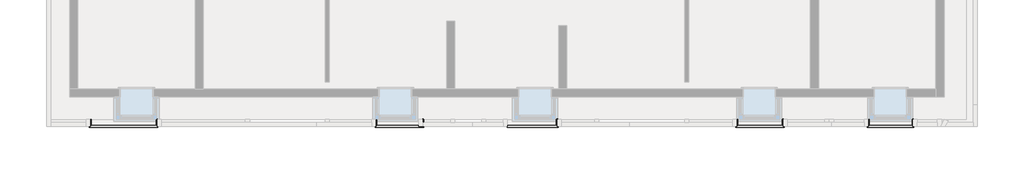
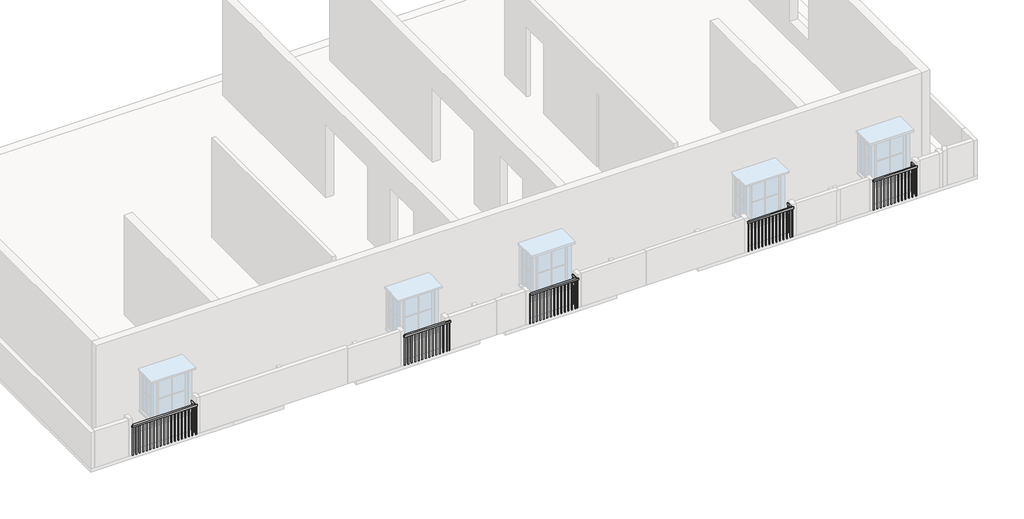
# One storey, part 3 of 7: 5 railings.
"""IFC4 building model written with IfcOpenShell, lengths in millimetres."""

from ifc_helpers import new_model, si_unit, frame, origin, place, context, project, spatial, polyline, outline, extrude, faceted_brep, element, save

model = new_model("IFC4")

# Units and contexts
model_context = context("Model", 3, world=origin())
ifc_project = project(units=[si_unit("LENGTHUNIT", "METRE", prefix="MILLI")], contexts=[model_context])

# Site, building, storey
site = spatial("IfcSite", under=ifc_project)
building = spatial("IfcBuilding", under=site)
storey = spatial("IfcBuildingStorey", under=building, Elevation=3200.4)

# Railings
placement = place(None, origin())
element("IfcRailing", 1, ObjectType="Handrail - Rectangular", at=placement, inside=storey, context=model_context, shape_type="SolidModel", body=[
    faceted_brep([(-11856.9067989, -4623.6932193, 4114.8), (-11856.9067989, -4623.6932193, 4064.0), (-11907.7067989, -4623.6932193, 4064.0), (-11907.7067989, -4623.6932193, 4114.8), (-11856.9067989, -4801.4932661, 4114.8), (-11856.9067989, -4801.4932661, 4064.0), (-11907.7067989, -4852.2932661, 4064.0), (-11907.7067989, -4852.2932661, 4114.8), (-10071.3470335, -4801.4932661, 4114.8), (-10071.3470335, -4801.4932661, 4064.0), (-10020.5470335, -4852.2932661, 4064.0), (-10020.5470335, -4852.2932661, 4114.8), (-10071.3470335, -4623.6932193, 4114.8), (-10020.5470335, -4623.6932193, 4114.8), (-10020.5470335, -4623.6932193, 4064.0), (-10071.3470335, -4623.6932193, 4064.0)], [[[0, 1, 2, 3]], [[1, 0, 4, 5]], [[2, 1, 5, 6]], [[3, 2, 6, 7]], [[0, 3, 7, 4]], [[5, 4, 8, 9]], [[6, 5, 9, 10]], [[7, 6, 10, 11]], [[4, 7, 11, 8]], [[12, 13, 14, 15]], [[9, 8, 12, 15]], [[10, 9, 15, 14]], [[11, 10, 14, 13]], [[8, 11, 13, 12]]]),
    extrude(outline(polyline([(-10036.4220335, -4633.2182661), (-10055.4720335, -4633.2182661), (-10055.4720335, -4614.1682661), (-10036.4220335, -4614.1682661), (-10036.4220335, -4633.2182661)])), frame((0.0, 0.0, 3200.4), z_axis=(0.0, 0.0, 1.0), x_axis=(1.0, 0.0, 0.0)), (0.0, 0.0, 1.0), 863.6),
    extrude(outline(polyline([(-10036.4220335, -4734.8182661), (-10055.4720335, -4734.8182661), (-10055.4720335, -4715.7682661), (-10036.4220335, -4715.7682661), (-10036.4220335, -4734.8182661)])), frame((0.0, 0.0, 3200.4), z_axis=(0.0, 0.0, 1.0), x_axis=(1.0, 0.0, 0.0)), (0.0, 0.0, 1.0), 863.6),
    extrude(outline(polyline([(-10063.0317989, -4836.4182661), (-10063.0317989, -4817.3682661), (-10043.9817989, -4817.3682661), (-10043.9817989, -4836.4182661), (-10063.0317989, -4836.4182661)])), frame((0.0, 0.0, 3200.4), z_axis=(0.0, 0.0, 1.0), x_axis=(1.0, 0.0, 0.0)), (0.0, 0.0, 1.0), 863.6),
    extrude(outline(polyline([(-10164.6317989, -4836.4182661), (-10164.6317989, -4817.3682661), (-10145.5817989, -4817.3682661), (-10145.5817989, -4836.4182661), (-10164.6317989, -4836.4182661)])), frame((0.0, 0.0, 3200.4), z_axis=(0.0, 0.0, 1.0), x_axis=(1.0, 0.0, 0.0)), (0.0, 0.0, 1.0), 863.6),
    extrude(outline(polyline([(-10266.2317989, -4836.4182661), (-10266.2317989, -4817.3682661), (-10247.1817989, -4817.3682661), (-10247.1817989, -4836.4182661), (-10266.2317989, -4836.4182661)])), frame((0.0, 0.0, 3200.4), z_axis=(0.0, 0.0, 1.0), x_axis=(1.0, 0.0, 0.0)), (0.0, 0.0, 1.0), 863.6),
    extrude(outline(polyline([(-10367.8317989, -4836.4182661), (-10367.8317989, -4817.3682661), (-10348.7817989, -4817.3682661), (-10348.7817989, -4836.4182661), (-10367.8317989, -4836.4182661)])), frame((0.0, 0.0, 3200.4), z_axis=(0.0, 0.0, 1.0), x_axis=(1.0, 0.0, 0.0)), (0.0, 0.0, 1.0), 863.6),
    extrude(outline(polyline([(-10469.4317989, -4836.4182661), (-10469.4317989, -4817.3682661), (-10450.3817989, -4817.3682661), (-10450.3817989, -4836.4182661), (-10469.4317989, -4836.4182661)])), frame((0.0, 0.0, 3200.4), z_axis=(0.0, 0.0, 1.0), x_axis=(1.0, 0.0, 0.0)), (0.0, 0.0, 1.0), 863.6),
    extrude(outline(polyline([(-10571.0317989, -4836.4182661), (-10571.0317989, -4817.3682661), (-10551.9817989, -4817.3682661), (-10551.9817989, -4836.4182661), (-10571.0317989, -4836.4182661)])), frame((0.0, 0.0, 3200.4), z_axis=(0.0, 0.0, 1.0), x_axis=(1.0, 0.0, 0.0)), (0.0, 0.0, 1.0), 863.6),
    extrude(outline(polyline([(-10672.6317989, -4836.4182661), (-10672.6317989, -4817.3682661), (-10653.5817989, -4817.3682661), (-10653.5817989, -4836.4182661), (-10672.6317989, -4836.4182661)])), frame((0.0, 0.0, 3200.4), z_axis=(0.0, 0.0, 1.0), x_axis=(1.0, 0.0, 0.0)), (0.0, 0.0, 1.0), 863.6),
    extrude(outline(polyline([(-10774.2317989, -4836.4182661), (-10774.2317989, -4817.3682661), (-10755.1817989, -4817.3682661), (-10755.1817989, -4836.4182661), (-10774.2317989, -4836.4182661)])), frame((0.0, 0.0, 3200.4), z_axis=(0.0, 0.0, 1.0), x_axis=(1.0, 0.0, 0.0)), (0.0, 0.0, 1.0), 863.6),
    extrude(outline(polyline([(-10875.8317989, -4836.4182661), (-10875.8317989, -4817.3682661), (-10856.7817989, -4817.3682661), (-10856.7817989, -4836.4182661), (-10875.8317989, -4836.4182661)])), frame((0.0, 0.0, 3200.4), z_axis=(0.0, 0.0, 1.0), x_axis=(1.0, 0.0, 0.0)), (0.0, 0.0, 1.0), 863.6),
    extrude(outline(polyline([(-10977.4317989, -4836.4182661), (-10977.4317989, -4817.3682661), (-10958.3817989, -4817.3682661), (-10958.3817989, -4836.4182661), (-10977.4317989, -4836.4182661)])), frame((0.0, 0.0, 3200.4), z_axis=(0.0, 0.0, 1.0), x_axis=(1.0, 0.0, 0.0)), (0.0, 0.0, 1.0), 863.6),
    extrude(outline(polyline([(-11079.0317989, -4836.4182661), (-11079.0317989, -4817.3682661), (-11059.9817989, -4817.3682661), (-11059.9817989, -4836.4182661), (-11079.0317989, -4836.4182661)])), frame((0.0, 0.0, 3200.4), z_axis=(0.0, 0.0, 1.0), x_axis=(1.0, 0.0, 0.0)), (0.0, 0.0, 1.0), 863.6),
    extrude(outline(polyline([(-11180.6317989, -4836.4182661), (-11180.6317989, -4817.3682661), (-11161.5817989, -4817.3682661), (-11161.5817989, -4836.4182661), (-11180.6317989, -4836.4182661)])), frame((0.0, 0.0, 3200.4), z_axis=(0.0, 0.0, 1.0), x_axis=(1.0, 0.0, 0.0)), (0.0, 0.0, 1.0), 863.6),
    extrude(outline(polyline([(-11282.2317989, -4836.4182661), (-11282.2317989, -4817.3682661), (-11263.1817989, -4817.3682661), (-11263.1817989, -4836.4182661), (-11282.2317989, -4836.4182661)])), frame((0.0, 0.0, 3200.4), z_axis=(0.0, 0.0, 1.0), x_axis=(1.0, 0.0, 0.0)), (0.0, 0.0, 1.0), 863.6),
    extrude(outline(polyline([(-11383.8317989, -4836.4182661), (-11383.8317989, -4817.3682661), (-11364.7817989, -4817.3682661), (-11364.7817989, -4836.4182661), (-11383.8317989, -4836.4182661)])), frame((0.0, 0.0, 3200.4), z_axis=(0.0, 0.0, 1.0), x_axis=(1.0, 0.0, 0.0)), (0.0, 0.0, 1.0), 863.6),
    extrude(outline(polyline([(-11485.4317989, -4836.4182661), (-11485.4317989, -4817.3682661), (-11466.3817989, -4817.3682661), (-11466.3817989, -4836.4182661), (-11485.4317989, -4836.4182661)])), frame((0.0, 0.0, 3200.4), z_axis=(0.0, 0.0, 1.0), x_axis=(1.0, 0.0, 0.0)), (0.0, 0.0, 1.0), 863.6),
    extrude(outline(polyline([(-11587.0317989, -4836.4182661), (-11587.0317989, -4817.3682661), (-11567.9817989, -4817.3682661), (-11567.9817989, -4836.4182661), (-11587.0317989, -4836.4182661)])), frame((0.0, 0.0, 3200.4), z_axis=(0.0, 0.0, 1.0), x_axis=(1.0, 0.0, 0.0)), (0.0, 0.0, 1.0), 863.6),
    extrude(outline(polyline([(-11688.6317989, -4836.4182661), (-11688.6317989, -4817.3682661), (-11669.5817989, -4817.3682661), (-11669.5817989, -4836.4182661), (-11688.6317989, -4836.4182661)])), frame((0.0, 0.0, 3200.4), z_axis=(0.0, 0.0, 1.0), x_axis=(1.0, 0.0, 0.0)), (0.0, 0.0, 1.0), 863.6),
    extrude(outline(polyline([(-11790.2317989, -4836.4182661), (-11790.2317989, -4817.3682661), (-11771.1817989, -4817.3682661), (-11771.1817989, -4836.4182661), (-11790.2317989, -4836.4182661)])), frame((0.0, 0.0, 3200.4), z_axis=(0.0, 0.0, 1.0), x_axis=(1.0, 0.0, 0.0)), (0.0, 0.0, 1.0), 863.6),
    extrude(outline(polyline([(-11891.8317989, -4817.3682193), (-11872.7817989, -4817.3682193), (-11872.7817989, -4836.4182193), (-11891.8317989, -4836.4182193), (-11891.8317989, -4817.3682193)])), frame((0.0, 0.0, 3200.4), z_axis=(0.0, 0.0, 1.0), x_axis=(1.0, 0.0, 0.0)), (0.0, 0.0, 1.0), 863.6),
    extrude(outline(polyline([(-11891.8317989, -4715.7682193), (-11872.7817989, -4715.7682193), (-11872.7817989, -4734.8182193), (-11891.8317989, -4734.8182193), (-11891.8317989, -4715.7682193)])), frame((0.0, 0.0, 3200.4), z_axis=(0.0, 0.0, 1.0), x_axis=(1.0, 0.0, 0.0)), (0.0, 0.0, 1.0), 863.6),
    extrude(outline(polyline([(-10055.4720335, -4836.4182661), (-10055.4720335, -4817.3682661), (-10036.4220335, -4817.3682661), (-10036.4220335, -4836.4182661), (-10055.4720335, -4836.4182661)])), frame((0.0, 0.0, 3200.4), z_axis=(0.0, 0.0, 1.0), x_axis=(1.0, 0.0, 0.0)), (0.0, 0.0, 1.0), 863.6),
    extrude(outline(polyline([(-11891.8317989, -4817.3682661), (-11872.7817989, -4817.3682661), (-11872.7817989, -4836.4182661), (-11891.8317989, -4836.4182661), (-11891.8317989, -4817.3682661)])), frame((0.0, 0.0, 3200.4), z_axis=(0.0, 0.0, 1.0), x_axis=(1.0, 0.0, 0.0)), (0.0, 0.0, 1.0), 863.6),
    extrude(outline(polyline([(-10036.4220335, -4642.7432193), (-10055.4720335, -4642.7432193), (-10055.4720335, -4623.6932193), (-10036.4220335, -4623.6932193), (-10036.4220335, -4642.7432193)])), frame((0.0, 0.0, 3200.4), z_axis=(0.0, 0.0, 1.0), x_axis=(1.0, 0.0, 0.0)), (0.0, 0.0, 1.0), 863.6),
    extrude(outline(polyline([(-11891.8317989, -4623.6932193), (-11872.7817989, -4623.6932193), (-11872.7817989, -4642.7432193), (-11891.8317989, -4642.7432193), (-11891.8317989, -4623.6932193)])), frame((0.0, 0.0, 3200.4), z_axis=(0.0, 0.0, 1.0), x_axis=(1.0, 0.0, 0.0)), (0.0, 0.0, 1.0), 863.6),
])
element("IfcRailing", 2, ObjectType="Handrail - Rectangular", at=placement, inside=storey, context=model_context, shape_type="SolidModel", body=[
    faceted_brep([(-3995.0987995, -4623.6932193, 4114.8), (-3995.0987995, -4623.6932193, 4064.0), (-4045.8987995, -4623.6932193, 4064.0), (-4045.8987995, -4623.6932193, 4114.8), (-3995.0987995, -4801.4932661, 4114.8), (-3995.0987995, -4801.4932661, 4064.0), (-4045.8987995, -4852.2932661, 4064.0), (-4045.8987995, -4852.2932661, 4114.8), (-2750.4987995, -4801.4932661, 4114.8), (-2750.4987995, -4801.4932661, 4064.0), (-2699.6987995, -4852.2932661, 4064.0), (-2699.6987995, -4852.2932661, 4114.8), (-2750.4987995, -4623.6932193, 4114.8), (-2699.6987995, -4623.6932193, 4114.8), (-2699.6987995, -4623.6932193, 4064.0), (-2750.4987995, -4623.6932193, 4064.0)], [[[0, 1, 2, 3]], [[1, 0, 4, 5]], [[2, 1, 5, 6]], [[3, 2, 6, 7]], [[0, 3, 7, 4]], [[5, 4, 8, 9]], [[6, 5, 9, 10]], [[7, 6, 10, 11]], [[4, 7, 11, 8]], [[12, 13, 14, 15]], [[9, 8, 12, 15]], [[10, 9, 15, 14]], [[11, 10, 14, 13]], [[8, 11, 13, 12]]]),
    extrude(outline(polyline([(-2715.5737995, -4633.2182661), (-2734.6237995, -4633.2182661), (-2734.6237995, -4614.1682661), (-2715.5737995, -4614.1682661), (-2715.5737995, -4633.2182661)])), frame((0.0, 0.0, 3200.4), z_axis=(0.0, 0.0, 1.0), x_axis=(1.0, 0.0, 0.0)), (0.0, 0.0, 1.0), 863.6),
    extrude(outline(polyline([(-2715.5737995, -4734.8182661), (-2734.6237995, -4734.8182661), (-2734.6237995, -4715.7682661), (-2715.5737995, -4715.7682661), (-2715.5737995, -4734.8182661)])), frame((0.0, 0.0, 3200.4), z_axis=(0.0, 0.0, 1.0), x_axis=(1.0, 0.0, 0.0)), (0.0, 0.0, 1.0), 863.6),
    extrude(outline(polyline([(-2810.8237995, -4836.4182661), (-2810.8237995, -4817.3682661), (-2791.7737995, -4817.3682661), (-2791.7737995, -4836.4182661), (-2810.8237995, -4836.4182661)])), frame((0.0, 0.0, 3200.4), z_axis=(0.0, 0.0, 1.0), x_axis=(1.0, 0.0, 0.0)), (0.0, 0.0, 1.0), 863.6),
    extrude(outline(polyline([(-2912.4237995, -4836.4182661), (-2912.4237995, -4817.3682661), (-2893.3737995, -4817.3682661), (-2893.3737995, -4836.4182661), (-2912.4237995, -4836.4182661)])), frame((0.0, 0.0, 3200.4), z_axis=(0.0, 0.0, 1.0), x_axis=(1.0, 0.0, 0.0)), (0.0, 0.0, 1.0), 863.6),
    extrude(outline(polyline([(-3014.0237995, -4836.4182661), (-3014.0237995, -4817.3682661), (-2994.9737995, -4817.3682661), (-2994.9737995, -4836.4182661), (-3014.0237995, -4836.4182661)])), frame((0.0, 0.0, 3200.4), z_axis=(0.0, 0.0, 1.0), x_axis=(1.0, 0.0, 0.0)), (0.0, 0.0, 1.0), 863.6),
    extrude(outline(polyline([(-3115.6237995, -4836.4182661), (-3115.6237995, -4817.3682661), (-3096.5737995, -4817.3682661), (-3096.5737995, -4836.4182661), (-3115.6237995, -4836.4182661)])), frame((0.0, 0.0, 3200.4), z_axis=(0.0, 0.0, 1.0), x_axis=(1.0, 0.0, 0.0)), (0.0, 0.0, 1.0), 863.6),
    extrude(outline(polyline([(-3217.2237995, -4836.4182661), (-3217.2237995, -4817.3682661), (-3198.1737995, -4817.3682661), (-3198.1737995, -4836.4182661), (-3217.2237995, -4836.4182661)])), frame((0.0, 0.0, 3200.4), z_axis=(0.0, 0.0, 1.0), x_axis=(1.0, 0.0, 0.0)), (0.0, 0.0, 1.0), 863.6),
    extrude(outline(polyline([(-3318.8237995, -4836.4182661), (-3318.8237995, -4817.3682661), (-3299.7737995, -4817.3682661), (-3299.7737995, -4836.4182661), (-3318.8237995, -4836.4182661)])), frame((0.0, 0.0, 3200.4), z_axis=(0.0, 0.0, 1.0), x_axis=(1.0, 0.0, 0.0)), (0.0, 0.0, 1.0), 863.6),
    extrude(outline(polyline([(-3420.4237995, -4836.4182661), (-3420.4237995, -4817.3682661), (-3401.3737995, -4817.3682661), (-3401.3737995, -4836.4182661), (-3420.4237995, -4836.4182661)])), frame((0.0, 0.0, 3200.4), z_axis=(0.0, 0.0, 1.0), x_axis=(1.0, 0.0, 0.0)), (0.0, 0.0, 1.0), 863.6),
    extrude(outline(polyline([(-3522.0237995, -4836.4182661), (-3522.0237995, -4817.3682661), (-3502.9737995, -4817.3682661), (-3502.9737995, -4836.4182661), (-3522.0237995, -4836.4182661)])), frame((0.0, 0.0, 3200.4), z_axis=(0.0, 0.0, 1.0), x_axis=(1.0, 0.0, 0.0)), (0.0, 0.0, 1.0), 863.6),
    extrude(outline(polyline([(-3623.6237995, -4836.4182661), (-3623.6237995, -4817.3682661), (-3604.5737995, -4817.3682661), (-3604.5737995, -4836.4182661), (-3623.6237995, -4836.4182661)])), frame((0.0, 0.0, 3200.4), z_axis=(0.0, 0.0, 1.0), x_axis=(1.0, 0.0, 0.0)), (0.0, 0.0, 1.0), 863.6),
    extrude(outline(polyline([(-3725.2237995, -4836.4182661), (-3725.2237995, -4817.3682661), (-3706.1737995, -4817.3682661), (-3706.1737995, -4836.4182661), (-3725.2237995, -4836.4182661)])), frame((0.0, 0.0, 3200.4), z_axis=(0.0, 0.0, 1.0), x_axis=(1.0, 0.0, 0.0)), (0.0, 0.0, 1.0), 863.6),
    extrude(outline(polyline([(-3826.8237995, -4836.4182661), (-3826.8237995, -4817.3682661), (-3807.7737995, -4817.3682661), (-3807.7737995, -4836.4182661), (-3826.8237995, -4836.4182661)])), frame((0.0, 0.0, 3200.4), z_axis=(0.0, 0.0, 1.0), x_axis=(1.0, 0.0, 0.0)), (0.0, 0.0, 1.0), 863.6),
    extrude(outline(polyline([(-3928.4237995, -4836.4182661), (-3928.4237995, -4817.3682661), (-3909.3737995, -4817.3682661), (-3909.3737995, -4836.4182661), (-3928.4237995, -4836.4182661)])), frame((0.0, 0.0, 3200.4), z_axis=(0.0, 0.0, 1.0), x_axis=(1.0, 0.0, 0.0)), (0.0, 0.0, 1.0), 863.6),
    extrude(outline(polyline([(-4030.0237995, -4817.3682193), (-4010.9737995, -4817.3682193), (-4010.9737995, -4836.4182193), (-4030.0237995, -4836.4182193), (-4030.0237995, -4817.3682193)])), frame((0.0, 0.0, 3200.4), z_axis=(0.0, 0.0, 1.0), x_axis=(1.0, 0.0, 0.0)), (0.0, 0.0, 1.0), 863.6),
    extrude(outline(polyline([(-4030.0237995, -4715.7682193), (-4010.9737995, -4715.7682193), (-4010.9737995, -4734.8182193), (-4030.0237995, -4734.8182193), (-4030.0237995, -4715.7682193)])), frame((0.0, 0.0, 3200.4), z_axis=(0.0, 0.0, 1.0), x_axis=(1.0, 0.0, 0.0)), (0.0, 0.0, 1.0), 863.6),
    extrude(outline(polyline([(-2734.6237995, -4836.4182661), (-2734.6237995, -4817.3682661), (-2715.5737995, -4817.3682661), (-2715.5737995, -4836.4182661), (-2734.6237995, -4836.4182661)])), frame((0.0, 0.0, 3200.4), z_axis=(0.0, 0.0, 1.0), x_axis=(1.0, 0.0, 0.0)), (0.0, 0.0, 1.0), 863.6),
    extrude(outline(polyline([(-4030.0237995, -4817.3682661), (-4010.9737995, -4817.3682661), (-4010.9737995, -4836.4182661), (-4030.0237995, -4836.4182661), (-4030.0237995, -4817.3682661)])), frame((0.0, 0.0, 3200.4), z_axis=(0.0, 0.0, 1.0), x_axis=(1.0, 0.0, 0.0)), (0.0, 0.0, 1.0), 863.6),
    extrude(outline(polyline([(-2715.5737995, -4642.7432193), (-2734.6237995, -4642.7432193), (-2734.6237995, -4623.6932193), (-2715.5737995, -4623.6932193), (-2715.5737995, -4642.7432193)])), frame((0.0, 0.0, 3200.4), z_axis=(0.0, 0.0, 1.0), x_axis=(1.0, 0.0, 0.0)), (0.0, 0.0, 1.0), 863.6),
    extrude(outline(polyline([(-4030.0237995, -4623.6932193), (-4010.9737995, -4623.6932193), (-4010.9737995, -4642.7432193), (-4030.0237995, -4642.7432193), (-4030.0237995, -4623.6932193)])), frame((0.0, 0.0, 3200.4), z_axis=(0.0, 0.0, 1.0), x_axis=(1.0, 0.0, 0.0)), (0.0, 0.0, 1.0), 863.6),
])
element("IfcRailing", 3, ObjectType="Handrail - Rectangular", at=placement, inside=storey, context=model_context, shape_type="SolidModel", body=[
    faceted_brep([(-406.2065315, -4801.4932661, 4114.8), (-406.2065315, -4801.4932661, 4064.0), (-406.2065315, -4852.2932661, 4064.0), (-406.2065315, -4852.2932661, 4114.8), (944.6932011, -4801.4932661, 4114.8), (944.6932011, -4801.4932661, 4064.0), (995.4932011, -4852.2932661, 4064.0), (995.4932011, -4852.2932661, 4114.8), (944.6932011, -4623.6932193, 4114.8), (995.4932011, -4623.6932193, 4114.8), (995.4932011, -4623.6932193, 4064.0), (944.6932011, -4623.6932193, 4064.0)], [[[0, 1, 2, 3]], [[1, 0, 4, 5]], [[2, 1, 5, 6]], [[3, 2, 6, 7]], [[0, 3, 7, 4]], [[8, 9, 10, 11]], [[5, 4, 8, 11]], [[6, 5, 11, 10]], [[7, 6, 10, 9]], [[4, 7, 9, 8]]]),
    extrude(outline(polyline([(979.6182011, -4633.2182661), (960.5682011, -4633.2182661), (960.5682011, -4614.1682661), (979.6182011, -4614.1682661), (979.6182011, -4633.2182661)])), frame((0.0, 0.0, 3200.4), z_axis=(0.0, 0.0, 1.0), x_axis=(1.0, 0.0, 0.0)), (0.0, 0.0, 1.0), 863.6),
    extrude(outline(polyline([(979.6182011, -4734.8182661), (960.5682011, -4734.8182661), (960.5682011, -4715.7682661), (979.6182011, -4715.7682661), (979.6182011, -4734.8182661)])), frame((0.0, 0.0, 3200.4), z_axis=(0.0, 0.0, 1.0), x_axis=(1.0, 0.0, 0.0)), (0.0, 0.0, 1.0), 863.6),
    extrude(outline(polyline([(905.0684685, -4836.4182661), (905.0684685, -4817.3682661), (924.1184685, -4817.3682661), (924.1184685, -4836.4182661), (905.0684685, -4836.4182661)])), frame((0.0, 0.0, 3200.4), z_axis=(0.0, 0.0, 1.0), x_axis=(1.0, 0.0, 0.0)), (0.0, 0.0, 1.0), 863.6),
    extrude(outline(polyline([(803.4684685, -4836.4182661), (803.4684685, -4817.3682661), (822.5184685, -4817.3682661), (822.5184685, -4836.4182661), (803.4684685, -4836.4182661)])), frame((0.0, 0.0, 3200.4), z_axis=(0.0, 0.0, 1.0), x_axis=(1.0, 0.0, 0.0)), (0.0, 0.0, 1.0), 863.6),
    extrude(outline(polyline([(701.8684685, -4836.4182661), (701.8684685, -4817.3682661), (720.9184685, -4817.3682661), (720.9184685, -4836.4182661), (701.8684685, -4836.4182661)])), frame((0.0, 0.0, 3200.4), z_axis=(0.0, 0.0, 1.0), x_axis=(1.0, 0.0, 0.0)), (0.0, 0.0, 1.0), 863.6),
    extrude(outline(polyline([(600.2684685, -4836.4182661), (600.2684685, -4817.3682661), (619.3184685, -4817.3682661), (619.3184685, -4836.4182661), (600.2684685, -4836.4182661)])), frame((0.0, 0.0, 3200.4), z_axis=(0.0, 0.0, 1.0), x_axis=(1.0, 0.0, 0.0)), (0.0, 0.0, 1.0), 863.6),
    extrude(outline(polyline([(498.6684685, -4836.4182661), (498.6684685, -4817.3682661), (517.7184685, -4817.3682661), (517.7184685, -4836.4182661), (498.6684685, -4836.4182661)])), frame((0.0, 0.0, 3200.4), z_axis=(0.0, 0.0, 1.0), x_axis=(1.0, 0.0, 0.0)), (0.0, 0.0, 1.0), 863.6),
    extrude(outline(polyline([(397.0684685, -4836.4182661), (397.0684685, -4817.3682661), (416.1184685, -4817.3682661), (416.1184685, -4836.4182661), (397.0684685, -4836.4182661)])), frame((0.0, 0.0, 3200.4), z_axis=(0.0, 0.0, 1.0), x_axis=(1.0, 0.0, 0.0)), (0.0, 0.0, 1.0), 863.6),
    extrude(outline(polyline([(295.4684685, -4836.4182661), (295.4684685, -4817.3682661), (314.5184685, -4817.3682661), (314.5184685, -4836.4182661), (295.4684685, -4836.4182661)])), frame((0.0, 0.0, 3200.4), z_axis=(0.0, 0.0, 1.0), x_axis=(1.0, 0.0, 0.0)), (0.0, 0.0, 1.0), 863.6),
    extrude(outline(polyline([(193.8684685, -4836.4182661), (193.8684685, -4817.3682661), (212.9184685, -4817.3682661), (212.9184685, -4836.4182661), (193.8684685, -4836.4182661)])), frame((0.0, 0.0, 3200.4), z_axis=(0.0, 0.0, 1.0), x_axis=(1.0, 0.0, 0.0)), (0.0, 0.0, 1.0), 863.6),
    extrude(outline(polyline([(92.2684685, -4836.4182661), (92.2684685, -4817.3682661), (111.3184685, -4817.3682661), (111.3184685, -4836.4182661), (92.2684685, -4836.4182661)])), frame((0.0, 0.0, 3200.4), z_axis=(0.0, 0.0, 1.0), x_axis=(1.0, 0.0, 0.0)), (0.0, 0.0, 1.0), 863.6),
    extrude(outline(polyline([(-9.3315315, -4836.4182661), (-9.3315315, -4817.3682661), (9.7184685, -4817.3682661), (9.7184685, -4836.4182661), (-9.3315315, -4836.4182661)])), frame((0.0, 0.0, 3200.4), z_axis=(0.0, 0.0, 1.0), x_axis=(1.0, 0.0, 0.0)), (0.0, 0.0, 1.0), 863.6),
    extrude(outline(polyline([(-110.9315315, -4836.4182661), (-110.9315315, -4817.3682661), (-91.8815315, -4817.3682661), (-91.8815315, -4836.4182661), (-110.9315315, -4836.4182661)])), frame((0.0, 0.0, 3200.4), z_axis=(0.0, 0.0, 1.0), x_axis=(1.0, 0.0, 0.0)), (0.0, 0.0, 1.0), 863.6),
    extrude(outline(polyline([(-212.5315315, -4836.4182661), (-212.5315315, -4817.3682661), (-193.4815315, -4817.3682661), (-193.4815315, -4836.4182661), (-212.5315315, -4836.4182661)])), frame((0.0, 0.0, 3200.4), z_axis=(0.0, 0.0, 1.0), x_axis=(1.0, 0.0, 0.0)), (0.0, 0.0, 1.0), 863.6),
    extrude(outline(polyline([(-314.1315315, -4836.4182661), (-314.1315315, -4817.3682661), (-295.0815315, -4817.3682661), (-295.0815315, -4836.4182661), (-314.1315315, -4836.4182661)])), frame((0.0, 0.0, 3200.4), z_axis=(0.0, 0.0, 1.0), x_axis=(1.0, 0.0, 0.0)), (0.0, 0.0, 1.0), 863.6),
    extrude(outline(polyline([(960.5682011, -4836.4182661), (960.5682011, -4817.3682661), (979.6182011, -4817.3682661), (979.6182011, -4836.4182661), (960.5682011, -4836.4182661)])), frame((0.0, 0.0, 3200.4), z_axis=(0.0, 0.0, 1.0), x_axis=(1.0, 0.0, 0.0)), (0.0, 0.0, 1.0), 863.6),
    extrude(outline(polyline([(979.6182011, -4642.7432193), (960.5682011, -4642.7432193), (960.5682011, -4623.6932193), (979.6182011, -4623.6932193), (979.6182011, -4642.7432193)])), frame((0.0, 0.0, 3200.4), z_axis=(0.0, 0.0, 1.0), x_axis=(1.0, 0.0, 0.0)), (0.0, 0.0, 1.0), 863.6),
    extrude(outline(polyline([(-406.2065315, -4836.4182661), (-406.2065315, -4817.3682661), (-387.1565315, -4817.3682661), (-387.1565315, -4836.4182661), (-406.2065315, -4836.4182661)])), frame((0.0, 0.0, 3200.4), z_axis=(0.0, 0.0, 1.0), x_axis=(1.0, 0.0, 0.0)), (0.0, 0.0, 1.0), 863.6),
])
element("IfcRailing", 4, ObjectType="Handrail - Rectangular", at=placement, inside=storey, context=model_context, shape_type="SolidModel", body=[
    faceted_brep([(5942.6512082, -4623.6932193, 4114.8), (5942.6512082, -4623.6932193, 4064.0), (5891.8512082, -4623.6932193, 4064.0), (5891.8512082, -4623.6932193, 4114.8), (5942.6512082, -4801.4932661, 4114.8), (5942.6512082, -4801.4932661, 4064.0), (5891.8512082, -4852.2932661, 4064.0), (5891.8512082, -4852.2932661, 4114.8), (7164.9011643, -4801.4932661, 4114.8), (7164.9011643, -4801.4932661, 4064.0), (7215.7011643, -4852.2932661, 4064.0), (7215.7011643, -4852.2932661, 4114.8), (7164.9011643, -4623.6932193, 4114.8), (7215.7011643, -4623.6932193, 4114.8), (7215.7011643, -4623.6932193, 4064.0), (7164.9011643, -4623.6932193, 4064.0)], [[[0, 1, 2, 3]], [[1, 0, 4, 5]], [[2, 1, 5, 6]], [[3, 2, 6, 7]], [[0, 3, 7, 4]], [[5, 4, 8, 9]], [[6, 5, 9, 10]], [[7, 6, 10, 11]], [[4, 7, 11, 8]], [[12, 13, 14, 15]], [[9, 8, 12, 15]], [[10, 9, 15, 14]], [[11, 10, 14, 13]], [[8, 11, 13, 12]]]),
    extrude(outline(polyline([(7199.8261643, -4633.2182661), (7180.7761643, -4633.2182661), (7180.7761643, -4614.1682661), (7199.8261643, -4614.1682661), (7199.8261643, -4633.2182661)])), frame((0.0, 0.0, 3200.4), z_axis=(0.0, 0.0, 1.0), x_axis=(1.0, 0.0, 0.0)), (0.0, 0.0, 1.0), 863.6),
    extrude(outline(polyline([(7199.8261643, -4734.8182661), (7180.7761643, -4734.8182661), (7180.7761643, -4715.7682661), (7199.8261643, -4715.7682661), (7199.8261643, -4734.8182661)])), frame((0.0, 0.0, 3200.4), z_axis=(0.0, 0.0, 1.0), x_axis=(1.0, 0.0, 0.0)), (0.0, 0.0, 1.0), 863.6),
    extrude(outline(polyline([(7126.9262082, -4836.4182661), (7126.9262082, -4817.3682661), (7145.9762082, -4817.3682661), (7145.9762082, -4836.4182661), (7126.9262082, -4836.4182661)])), frame((0.0, 0.0, 3200.4), z_axis=(0.0, 0.0, 1.0), x_axis=(1.0, 0.0, 0.0)), (0.0, 0.0, 1.0), 863.6),
    extrude(outline(polyline([(7025.3262082, -4836.4182661), (7025.3262082, -4817.3682661), (7044.3762082, -4817.3682661), (7044.3762082, -4836.4182661), (7025.3262082, -4836.4182661)])), frame((0.0, 0.0, 3200.4), z_axis=(0.0, 0.0, 1.0), x_axis=(1.0, 0.0, 0.0)), (0.0, 0.0, 1.0), 863.6),
    extrude(outline(polyline([(6923.7262082, -4836.4182661), (6923.7262082, -4817.3682661), (6942.7762082, -4817.3682661), (6942.7762082, -4836.4182661), (6923.7262082, -4836.4182661)])), frame((0.0, 0.0, 3200.4), z_axis=(0.0, 0.0, 1.0), x_axis=(1.0, 0.0, 0.0)), (0.0, 0.0, 1.0), 863.6),
    extrude(outline(polyline([(6822.1262082, -4836.4182661), (6822.1262082, -4817.3682661), (6841.1762082, -4817.3682661), (6841.1762082, -4836.4182661), (6822.1262082, -4836.4182661)])), frame((0.0, 0.0, 3200.4), z_axis=(0.0, 0.0, 1.0), x_axis=(1.0, 0.0, 0.0)), (0.0, 0.0, 1.0), 863.6),
    extrude(outline(polyline([(6720.5262082, -4836.4182661), (6720.5262082, -4817.3682661), (6739.5762082, -4817.3682661), (6739.5762082, -4836.4182661), (6720.5262082, -4836.4182661)])), frame((0.0, 0.0, 3200.4), z_axis=(0.0, 0.0, 1.0), x_axis=(1.0, 0.0, 0.0)), (0.0, 0.0, 1.0), 863.6),
    extrude(outline(polyline([(6618.9262082, -4836.4182661), (6618.9262082, -4817.3682661), (6637.9762082, -4817.3682661), (6637.9762082, -4836.4182661), (6618.9262082, -4836.4182661)])), frame((0.0, 0.0, 3200.4), z_axis=(0.0, 0.0, 1.0), x_axis=(1.0, 0.0, 0.0)), (0.0, 0.0, 1.0), 863.6),
    extrude(outline(polyline([(6517.3262082, -4836.4182661), (6517.3262082, -4817.3682661), (6536.3762082, -4817.3682661), (6536.3762082, -4836.4182661), (6517.3262082, -4836.4182661)])), frame((0.0, 0.0, 3200.4), z_axis=(0.0, 0.0, 1.0), x_axis=(1.0, 0.0, 0.0)), (0.0, 0.0, 1.0), 863.6),
    extrude(outline(polyline([(6415.7262082, -4836.4182661), (6415.7262082, -4817.3682661), (6434.7762082, -4817.3682661), (6434.7762082, -4836.4182661), (6415.7262082, -4836.4182661)])), frame((0.0, 0.0, 3200.4), z_axis=(0.0, 0.0, 1.0), x_axis=(1.0, 0.0, 0.0)), (0.0, 0.0, 1.0), 863.6),
    extrude(outline(polyline([(6314.1262082, -4836.4182661), (6314.1262082, -4817.3682661), (6333.1762082, -4817.3682661), (6333.1762082, -4836.4182661), (6314.1262082, -4836.4182661)])), frame((0.0, 0.0, 3200.4), z_axis=(0.0, 0.0, 1.0), x_axis=(1.0, 0.0, 0.0)), (0.0, 0.0, 1.0), 863.6),
    extrude(outline(polyline([(6212.5262082, -4836.4182661), (6212.5262082, -4817.3682661), (6231.5762082, -4817.3682661), (6231.5762082, -4836.4182661), (6212.5262082, -4836.4182661)])), frame((0.0, 0.0, 3200.4), z_axis=(0.0, 0.0, 1.0), x_axis=(1.0, 0.0, 0.0)), (0.0, 0.0, 1.0), 863.6),
    extrude(outline(polyline([(6110.9262082, -4836.4182661), (6110.9262082, -4817.3682661), (6129.9762082, -4817.3682661), (6129.9762082, -4836.4182661), (6110.9262082, -4836.4182661)])), frame((0.0, 0.0, 3200.4), z_axis=(0.0, 0.0, 1.0), x_axis=(1.0, 0.0, 0.0)), (0.0, 0.0, 1.0), 863.6),
    extrude(outline(polyline([(6009.3262082, -4836.4182661), (6009.3262082, -4817.3682661), (6028.3762082, -4817.3682661), (6028.3762082, -4836.4182661), (6009.3262082, -4836.4182661)])), frame((0.0, 0.0, 3200.4), z_axis=(0.0, 0.0, 1.0), x_axis=(1.0, 0.0, 0.0)), (0.0, 0.0, 1.0), 863.6),
    extrude(outline(polyline([(5907.7262082, -4817.3682193), (5926.7762082, -4817.3682193), (5926.7762082, -4836.4182193), (5907.7262082, -4836.4182193), (5907.7262082, -4817.3682193)])), frame((0.0, 0.0, 3200.4), z_axis=(0.0, 0.0, 1.0), x_axis=(1.0, 0.0, 0.0)), (0.0, 0.0, 1.0), 863.6),
    extrude(outline(polyline([(5907.7262082, -4715.7682193), (5926.7762082, -4715.7682193), (5926.7762082, -4734.8182193), (5907.7262082, -4734.8182193), (5907.7262082, -4715.7682193)])), frame((0.0, 0.0, 3200.4), z_axis=(0.0, 0.0, 1.0), x_axis=(1.0, 0.0, 0.0)), (0.0, 0.0, 1.0), 863.6),
    extrude(outline(polyline([(7180.7761643, -4836.4182661), (7180.7761643, -4817.3682661), (7199.8261643, -4817.3682661), (7199.8261643, -4836.4182661), (7180.7761643, -4836.4182661)])), frame((0.0, 0.0, 3200.4), z_axis=(0.0, 0.0, 1.0), x_axis=(1.0, 0.0, 0.0)), (0.0, 0.0, 1.0), 863.6),
    extrude(outline(polyline([(5907.7262082, -4817.3682661), (5926.7762082, -4817.3682661), (5926.7762082, -4836.4182661), (5907.7262082, -4836.4182661), (5907.7262082, -4817.3682661)])), frame((0.0, 0.0, 3200.4), z_axis=(0.0, 0.0, 1.0), x_axis=(1.0, 0.0, 0.0)), (0.0, 0.0, 1.0), 863.6),
    extrude(outline(polyline([(7199.8261643, -4642.7432193), (7180.7761643, -4642.7432193), (7180.7761643, -4623.6932193), (7199.8261643, -4623.6932193), (7199.8261643, -4642.7432193)])), frame((0.0, 0.0, 3200.4), z_axis=(0.0, 0.0, 1.0), x_axis=(1.0, 0.0, 0.0)), (0.0, 0.0, 1.0), 863.6),
    extrude(outline(polyline([(5907.7262082, -4623.6932193), (5926.7762082, -4623.6932193), (5926.7762082, -4642.7432193), (5907.7262082, -4642.7432193), (5907.7262082, -4623.6932193)])), frame((0.0, 0.0, 3200.4), z_axis=(0.0, 0.0, 1.0), x_axis=(1.0, 0.0, 0.0)), (0.0, 0.0, 1.0), 863.6),
])
element("IfcRailing", 5, ObjectType="Handrail - Rectangular", at=placement, inside=storey, context=model_context, shape_type="SolidModel", body=[
    faceted_brep([(9562.1512082, -4623.6932193, 4114.8), (9562.1512082, -4623.6932193, 4064.0), (9511.3512082, -4623.6932193, 4064.0), (9511.3512082, -4623.6932193, 4114.8), (9562.1512082, -4801.4932661, 4114.8), (9562.1512082, -4801.4932661, 4064.0), (9511.3512082, -4852.2932661, 4064.0), (9511.3512082, -4852.2932661, 4114.8), (10738.7617205, -4801.4932661, 4114.8), (10738.7617205, -4801.4932661, 4064.0), (10789.5617205, -4852.2932661, 4064.0), (10789.5617205, -4852.2932661, 4114.8), (10738.7617205, -4623.6932193, 4114.8), (10789.5617205, -4623.6932193, 4114.8), (10789.5617205, -4623.6932193, 4064.0), (10738.7617205, -4623.6932193, 4064.0)], [[[0, 1, 2, 3]], [[1, 0, 4, 5]], [[2, 1, 5, 6]], [[3, 2, 6, 7]], [[0, 3, 7, 4]], [[5, 4, 8, 9]], [[6, 5, 9, 10]], [[7, 6, 10, 11]], [[4, 7, 11, 8]], [[12, 13, 14, 15]], [[9, 8, 12, 15]], [[10, 9, 15, 14]], [[11, 10, 14, 13]], [[8, 11, 13, 12]]]),
    extrude(outline(polyline([(10754.6367205, -4633.2182661), (10754.6367205, -4614.1682661), (10773.6867205, -4614.1682661), (10773.6867205, -4633.2182661), (10754.6367205, -4633.2182661)])), frame((0.0, 0.0, 3200.4), z_axis=(0.0, 0.0, 1.0), x_axis=(1.0, 0.0, 0.0)), (0.0, 0.0, 1.0), 863.6),
    extrude(outline(polyline([(10754.6367205, -4734.8182661), (10754.6367205, -4715.7682661), (10773.6867205, -4715.7682661), (10773.6867205, -4734.8182661), (10754.6367205, -4734.8182661)])), frame((0.0, 0.0, 3200.4), z_axis=(0.0, 0.0, 1.0), x_axis=(1.0, 0.0, 0.0)), (0.0, 0.0, 1.0), 863.6),
    extrude(outline(polyline([(10746.4262082, -4817.3682661), (10765.4762082, -4817.3682661), (10765.4762082, -4836.4182661), (10746.4262082, -4836.4182661), (10746.4262082, -4817.3682661)])), frame((0.0, 0.0, 3200.4), z_axis=(0.0, 0.0, 1.0), x_axis=(1.0, 0.0, 0.0)), (0.0, 0.0, 1.0), 863.6),
    extrude(outline(polyline([(10644.8262082, -4817.3682661), (10663.8762082, -4817.3682661), (10663.8762082, -4836.4182661), (10644.8262082, -4836.4182661), (10644.8262082, -4817.3682661)])), frame((0.0, 0.0, 3200.4), z_axis=(0.0, 0.0, 1.0), x_axis=(1.0, 0.0, 0.0)), (0.0, 0.0, 1.0), 863.6),
    extrude(outline(polyline([(10543.2262082, -4817.3682661), (10562.2762082, -4817.3682661), (10562.2762082, -4836.4182661), (10543.2262082, -4836.4182661), (10543.2262082, -4817.3682661)])), frame((0.0, 0.0, 3200.4), z_axis=(0.0, 0.0, 1.0), x_axis=(1.0, 0.0, 0.0)), (0.0, 0.0, 1.0), 863.6),
    extrude(outline(polyline([(10441.6262082, -4817.3682661), (10460.6762082, -4817.3682661), (10460.6762082, -4836.4182661), (10441.6262082, -4836.4182661), (10441.6262082, -4817.3682661)])), frame((0.0, 0.0, 3200.4), z_axis=(0.0, 0.0, 1.0), x_axis=(1.0, 0.0, 0.0)), (0.0, 0.0, 1.0), 863.6),
    extrude(outline(polyline([(10340.0262082, -4817.3682661), (10359.0762082, -4817.3682661), (10359.0762082, -4836.4182661), (10340.0262082, -4836.4182661), (10340.0262082, -4817.3682661)])), frame((0.0, 0.0, 3200.4), z_axis=(0.0, 0.0, 1.0), x_axis=(1.0, 0.0, 0.0)), (0.0, 0.0, 1.0), 863.6),
    extrude(outline(polyline([(10238.4262082, -4817.3682661), (10257.4762082, -4817.3682661), (10257.4762082, -4836.4182661), (10238.4262082, -4836.4182661), (10238.4262082, -4817.3682661)])), frame((0.0, 0.0, 3200.4), z_axis=(0.0, 0.0, 1.0), x_axis=(1.0, 0.0, 0.0)), (0.0, 0.0, 1.0), 863.6),
    extrude(outline(polyline([(10136.8262082, -4817.3682661), (10155.8762082, -4817.3682661), (10155.8762082, -4836.4182661), (10136.8262082, -4836.4182661), (10136.8262082, -4817.3682661)])), frame((0.0, 0.0, 3200.4), z_axis=(0.0, 0.0, 1.0), x_axis=(1.0, 0.0, 0.0)), (0.0, 0.0, 1.0), 863.6),
    extrude(outline(polyline([(10035.2262082, -4817.3682661), (10054.2762082, -4817.3682661), (10054.2762082, -4836.4182661), (10035.2262082, -4836.4182661), (10035.2262082, -4817.3682661)])), frame((0.0, 0.0, 3200.4), z_axis=(0.0, 0.0, 1.0), x_axis=(1.0, 0.0, 0.0)), (0.0, 0.0, 1.0), 863.6),
    extrude(outline(polyline([(9933.6262082, -4817.3682661), (9952.6762082, -4817.3682661), (9952.6762082, -4836.4182661), (9933.6262082, -4836.4182661), (9933.6262082, -4817.3682661)])), frame((0.0, 0.0, 3200.4), z_axis=(0.0, 0.0, 1.0), x_axis=(1.0, 0.0, 0.0)), (0.0, 0.0, 1.0), 863.6),
    extrude(outline(polyline([(9832.0262082, -4817.3682661), (9851.0762082, -4817.3682661), (9851.0762082, -4836.4182661), (9832.0262082, -4836.4182661), (9832.0262082, -4817.3682661)])), frame((0.0, 0.0, 3200.4), z_axis=(0.0, 0.0, 1.0), x_axis=(1.0, 0.0, 0.0)), (0.0, 0.0, 1.0), 863.6),
    extrude(outline(polyline([(9730.4262082, -4817.3682661), (9749.4762082, -4817.3682661), (9749.4762082, -4836.4182661), (9730.4262082, -4836.4182661), (9730.4262082, -4817.3682661)])), frame((0.0, 0.0, 3200.4), z_axis=(0.0, 0.0, 1.0), x_axis=(1.0, 0.0, 0.0)), (0.0, 0.0, 1.0), 863.6),
    extrude(outline(polyline([(9628.8262082, -4817.3682661), (9647.8762082, -4817.3682661), (9647.8762082, -4836.4182661), (9628.8262082, -4836.4182661), (9628.8262082, -4817.3682661)])), frame((0.0, 0.0, 3200.4), z_axis=(0.0, 0.0, 1.0), x_axis=(1.0, 0.0, 0.0)), (0.0, 0.0, 1.0), 863.6),
    extrude(outline(polyline([(9546.2762082, -4817.3682193), (9546.2762082, -4836.4182193), (9527.2262082, -4836.4182193), (9527.2262082, -4817.3682193), (9546.2762082, -4817.3682193)])), frame((0.0, 0.0, 3200.4), z_axis=(0.0, 0.0, 1.0), x_axis=(1.0, 0.0, 0.0)), (0.0, 0.0, 1.0), 863.6),
    extrude(outline(polyline([(9546.2762082, -4715.7682193), (9546.2762082, -4734.8182193), (9527.2262082, -4734.8182193), (9527.2262082, -4715.7682193), (9546.2762082, -4715.7682193)])), frame((0.0, 0.0, 3200.4), z_axis=(0.0, 0.0, 1.0), x_axis=(1.0, 0.0, 0.0)), (0.0, 0.0, 1.0), 863.6),
    extrude(outline(polyline([(10754.6367205, -4817.3682661), (10773.6867205, -4817.3682661), (10773.6867205, -4836.4182661), (10754.6367205, -4836.4182661), (10754.6367205, -4817.3682661)])), frame((0.0, 0.0, 3200.4), z_axis=(0.0, 0.0, 1.0), x_axis=(1.0, 0.0, 0.0)), (0.0, 0.0, 1.0), 863.6),
    extrude(outline(polyline([(9546.2762082, -4817.3682661), (9546.2762082, -4836.4182661), (9527.2262082, -4836.4182661), (9527.2262082, -4817.3682661), (9546.2762082, -4817.3682661)])), frame((0.0, 0.0, 3200.4), z_axis=(0.0, 0.0, 1.0), x_axis=(1.0, 0.0, 0.0)), (0.0, 0.0, 1.0), 863.6),
    extrude(outline(polyline([(10754.6367205, -4642.7432193), (10754.6367205, -4623.6932193), (10773.6867205, -4623.6932193), (10773.6867205, -4642.7432193), (10754.6367205, -4642.7432193)])), frame((0.0, 0.0, 3200.4), z_axis=(0.0, 0.0, 1.0), x_axis=(1.0, 0.0, 0.0)), (0.0, 0.0, 1.0), 863.6),
    extrude(outline(polyline([(9546.2762082, -4623.6932193), (9546.2762082, -4642.7432193), (9527.2262082, -4642.7432193), (9527.2262082, -4623.6932193), (9546.2762082, -4623.6932193)])), frame((0.0, 0.0, 3200.4), z_axis=(0.0, 0.0, 1.0), x_axis=(1.0, 0.0, 0.0)), (0.0, 0.0, 1.0), 863.6),
])

save(model, "model.ifc")

# Revit data of these elements
# Type "Handrail - Rectangular"
#   Assembly Code = "C2010400"
#   built-in parameter 1008612 = 0.0416667 (stored number, unit not read)
#   built-in parameter 1008611 = 0.0416667 (stored number, unit not read)
#   built-in parameter 1008609 = 0.333333 (stored number, unit not read)
#   built-in parameter 1008604 = 0.166667 (stored number, unit not read)
#   built-in parameter 1008603 = 0.166667 (stored number, unit not read)
#   Railing Height = 3' - 0"
#   built-in parameter 1008630 = 2
#   built-in parameter 1008610 = 2
#   built-in parameter 1008618 = Baluster - Square : 3/4"
# Elements 1, 2, 3, 4, 5 (IfcRailing, "Handrail - Rectangular")
#   Phase Created = New Construction
